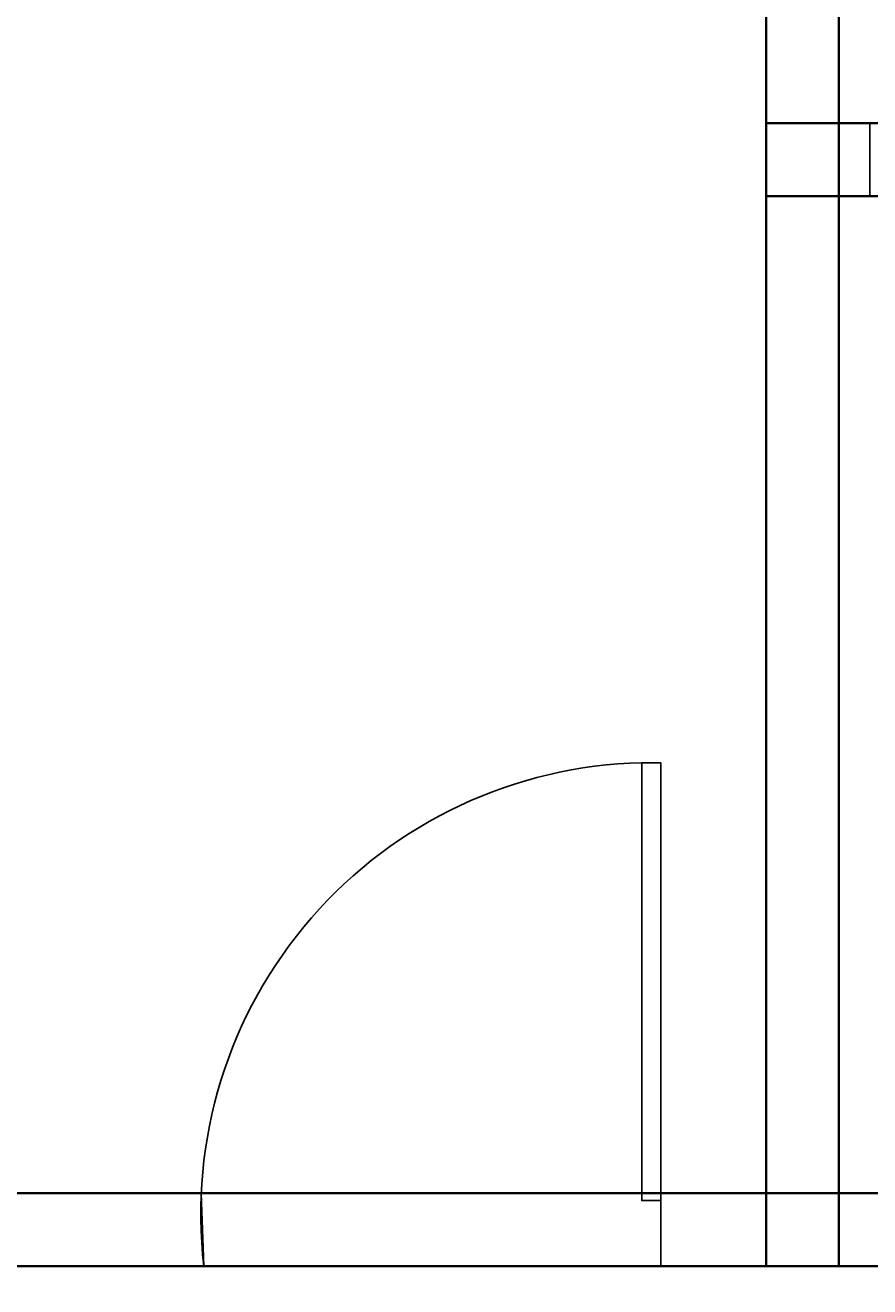
# Model space of a CAD drawing. Units: inches. Extents: x -61 to 1599, y -1316 to 257.
# Tile 40 of 204: x 171 to 240, y -790 to -686. Entities that reach past the tile are written whole.
import ezdxf

# ---------------------------------------------------------------- set-up
doc = ezdxf.new("R2010")
doc.units = ezdxf.units.IN
doc.header["$MEASUREMENT"] = 0
doc.linetypes.add('ACAD_ISO02W100', pattern=[15, 12, -3])
for name, color, linetype, lineweight in [('A-ANNO-DIMS', 2, 'Continuous', 18), ('A-WALL-JAMB', 4, 'ACAD_ISO02W100', 25), ('DOORS', 2, 'Continuous', 25), ('WALLS', 4, 'Continuous', 35)]:
    doc.layers.add(name, color=color, linetype=linetype, lineweight=lineweight)
doc.styles.get("Standard").update_dxf_attribs({"font": 'arial.ttf'})
doc.dimstyles.get("Standard").update_dxf_attribs({"dimtxt": 0.18, "dimasz": 0.18, "dimexe": 0.18, "dimexo": 0.0625, "dimgap": 0.09, "dimtad": 0, "dimtih": 1, "dimtoh": 1, "dimdec": 0, "dimzin": 0, "dimdsep": 46, "dimlunit": 3, "dimtxsty": 'Standard', "dimcen": 0.09, "dimadec": 0, "dimazin": 0, "dimtfac": 1, "dimtdec": 0, "dimtofl": 0, "dimtmove": 0, "dimatfit": 3, "dimfxl": 1, "dimtolj": 1, "dimtzin": 0, "dimarcsym": 0})

# ---------------------------------------------------------------- blocks, each defined once
blk = doc.blocks.new('DOOR-SWING-36')
blk.add_line((0, 0), (0, -5.4))
blk.add_lwpolyline([(0, 0), (0, 36), (-1.57, 36), (-1.57, 0)], close=True)
blk.add_arc((-0.74, -1.08), 37.09, 91.2913, 186.6905)
blk = doc.blocks.new('*D687')
at = {"layer": 'A-ANNO-DIMS', "color": 0, "lineweight": -2, "transparency": 16777216}
for p, q in [((289.42, 181.68), (-61.08, 181.68)), ((-60.9, 181.5), (-60.9, -528.95)), ((-60.9, -1239.76), (-60.9, -529.32)), ((319.64, -1239.94), (-61.08, -1239.94))]:
    blk.add_line(p, q, dxfattribs=at)
at = {"layer": 'A-ANNO-DIMS', "color": 0, "transparency": 16777216}
for points in [[(-60.93, 181.5), (-60.87, 181.5), (-60.9, 181.68)], [(-60.93, -1239.76), (-60.87, -1239.76), (-60.9, -1239.94)]]:
    blk.add_solid(points, dxfattribs=at)
at = {"layer": 'DEFPOINTS', "color": 0, "transparency": 16777216}
for p in [(289.48, 181.68), (-60.9, -1239.94), (319.7, -1239.94)]:
    blk.add_point(p, dxfattribs=at)
at = {"layer": 'A-ANNO-DIMS', "color": 0, "transparency": 16777216, "insert": (-60.9, -529.13), "char_height": 0.18, "attachment_point": 5}
blk.add_mtext('\\A1;1421.6', dxfattribs=at)

msp = doc.modelspace()

# ---------------------------------------------------------------- linework, layer by layer
at = {"layer": 'A-WALL-JAMB'}
for p, q in [((240.2351, -693.9446), (240.2351, -699.9446)), ((185.4756, -787.9446), (185.2611, -781.9446)), ((223.0506, -787.9446), (223.0506, -781.9446))]:
    msp.add_line(p, q, dxfattribs=at)
at = {"layer": 'WALLS'}
for p, q in [((231.7028, -616.9446), (231.7028, -787.9446)), ((237.7028, -616.9446), (237.7028, -787.9446)), ((231.7028, -693.9446), (327.7028, -693.9446)), ((231.7028, -699.9446), (327.7028, -699.9446)), ((14.7028, -781.9446), (237.7028, -781.9446)), ((237.7028, -781.9446), (327.7028, -781.9446)), ((14.7028, -787.9446), (237.7028, -787.9446)), ((237.7028, -787.9446), (327.7028, -787.9446))]:
    msp.add_line(p, q, dxfattribs=at)

# ---------------------------------------------------------------- block references
at = {"layer": 'DOORS'}
msp.add_blockref('DOOR-SWING-36', (223.0506, -782.5446), dxfattribs=at)

# ---------------------------------------------------------------- dimensions: what is measured, and where the dimension line sits
at = {"layer": 'A-ANNO-DIMS'}
dim = msp.add_linear_dim(base=(-60.8972, -1239.9446), p1=(289.4807, 181.6771), p2=(319.7028, -1239.9446), angle=90, dimstyle='Standard', override={"dimdec": 1, "dimlfac": 1, "dimrnd": 0, "dimzin": 0, "dimdsep": 46, "dimlunit": 2}, dxfattribs=at)
dim.commit()
dim.dimension.update_dxf_attribs({"geometry": '*D687', "text_midpoint": (-60.8972, -529.1337)})

doc.saveas('drawing.dxf')
